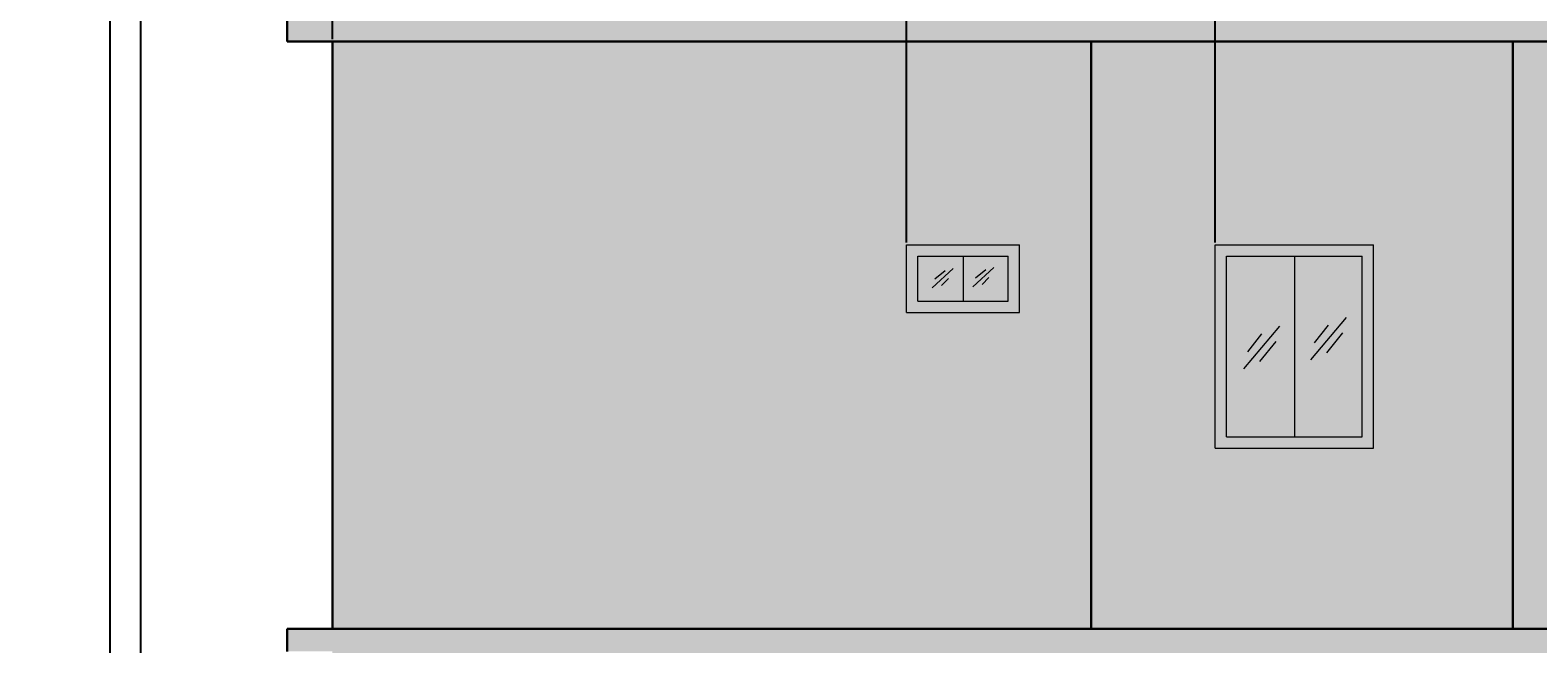
# Model space of a CAD drawing. Units: inches. Extents: x 2391 to 16591, y 7259 to 10239.
# Tile 14 of 27: x 3487 to 3888, y 8066 to 8229. Entities that reach past the tile are written whole.
import ezdxf

# ---------------------------------------------------------------- set-up
doc = ezdxf.new("R2010")
doc.units = ezdxf.units.IN
for name, color, linetype, lineweight in [('A-ANNO-DIMS', 4, 'Continuous', 18), ('A-ELEV', 7, 'Continuous', 30), ('A-ELEV-GLAZ', 4, 'Continuous', 18), ('A-ELEV-GLAZ-PATT', 141, 'Continuous', 13), ('A-ELEV-PATT', 8, 'Continuous', 13), ('A-ELEV-SURF-PATT', 253, 'Continuous', 13)]:
    doc.layers.add(name, color=color, linetype=linetype, lineweight=lineweight)
doc.styles.get("Standard").update_dxf_attribs({"font": 'arial.ttf'})
doc.dimstyles.new('ISO-25', dxfattribs={"dimtxt": 2.5, "dimasz": 2.5, "dimexe": 1.25, "dimexo": 0.625, "dimtad": 1, "dimdec": 0, "dimlunit": 3, "dimtxsty": 'Standard', "dimcen": 2.5, "dimadec": 0, "dimazin": 0, "dimtfac": 1, "dimtdec": 0, "dimtmove": 0, "dimatfit": 3, "dimfxl": 1, "dimarcsym": 0})

# ---------------------------------------------------------------- blocks, each defined once
blk = doc.blocks.new('GLASS-REFLECTION-VENT')
for p, q in [((0, 0), (5.55, 5.12)), ((0.7, 2.37), (3.45, 4.58)), ((2.48, 0.59), (4.26, 2.48))]:
    blk.add_line(p, q)
blk = doc.blocks.new('GLASS-REFLECTION-WINDOW')
for p, q in [((0, 0), (9.5, 11.3)), ((1, 4.52), (4.76, 9.26)), ((4.26, 1.91), (8.52, 7.21))]:
    blk.add_line(p, q)
blk = doc.blocks.new('*D84')
at = {"layer": 'A-ANNO-DIMS', "color": 0, "lineweight": -2, "transparency": 16777216}
for p, q in [((3437.4, 8339.52), (3518.08, 8339.52)), ((3516.83, 7579.02), (3516.83, 8337.02)), ((3464.4, 7576.52), (3518.08, 7576.52))]:
    blk.add_line(p, q, dxfattribs=at)
at = {"layer": 'A-ANNO-DIMS', "color": 0, "transparency": 16777216}
for points in [[(3516.41, 8337.02), (3517.24, 8337.02), (3516.83, 8339.52)], [(3516.41, 7579.02), (3517.24, 7579.02), (3516.83, 7576.52)]]:
    blk.add_solid(points, dxfattribs=at)
at = {"layer": 'Defpoints', "color": 0, "transparency": 16777216}
for p in [(3436.78, 8339.52), (3516.83, 8339.52), (3463.78, 7576.52)]:
    blk.add_point(p, dxfattribs=at)
at = {"layer": 'A-ANNO-DIMS', "color": 0, "transparency": 16777216, "insert": (3514.93, 7958.02), "char_height": 2.5, "attachment_point": 5, "rotation": 90}
blk.add_mtext('63\'-7"', dxfattribs=at)
blk = doc.blocks.new('*D92')
at = {"layer": 'A-ANNO-DIMS', "color": 0, "lineweight": -2, "transparency": 16777216}
for p, q in [((3777.58, 8333.18), (3507.41, 8333.18)), ((3508.66, 7572.68), (3508.66, 8330.68)), ((3561.08, 7570.18), (3507.41, 7570.18))]:
    blk.add_line(p, q, dxfattribs=at)
at = {"layer": 'A-ANNO-DIMS', "color": 0, "transparency": 16777216}
for points in [[(3508.24, 8330.68), (3509.08, 8330.68), (3508.66, 8333.18)], [(3508.24, 7572.68), (3509.08, 7572.68), (3508.66, 7570.18)]]:
    blk.add_solid(points, dxfattribs=at)
at = {"layer": 'Defpoints', "color": 0, "transparency": 16777216}
for p in [(3508.66, 8333.18), (3778.21, 8333.18), (3561.71, 7570.18)]:
    blk.add_point(p, dxfattribs=at)
at = {"layer": 'A-ANNO-DIMS', "color": 0, "transparency": 16777216, "insert": (3506.76, 7951.68), "char_height": 2.5, "attachment_point": 5, "rotation": 90}
blk.add_mtext('63\'-7"', dxfattribs=at)
blk = doc.blocks.new('*D93')
at = {"layer": 'A-ANNO-DIMS', "color": 0, "lineweight": -2, "transparency": 16777216}
for p, q in [((3567.71, 8226.81), (3567.71, 8381.48)), ((3570.21, 8380.23), (3717.71, 8380.23)), ((3720.21, 8172.81), (3720.21, 8381.48))]:
    blk.add_line(p, q, dxfattribs=at)
at = {"layer": 'A-ANNO-DIMS', "color": 0, "transparency": 16777216}
for points in [[(3570.21, 8380.65), (3570.21, 8379.81), (3567.71, 8380.23)], [(3717.71, 8380.65), (3717.71, 8379.81), (3720.21, 8380.23)]]:
    blk.add_solid(points, dxfattribs=at)
at = {"layer": 'Defpoints', "color": 0, "transparency": 16777216}
for p in [(3720.21, 8380.23), (3567.71, 8226.18), (3720.21, 8172.18)]:
    blk.add_point(p, dxfattribs=at)
at = {"layer": 'A-ANNO-DIMS', "color": 0, "transparency": 16777216, "insert": (3643.96, 8382.15), "char_height": 2.5, "attachment_point": 5}
blk.add_mtext('12\'-8 1/2"', dxfattribs=at)
blk = doc.blocks.new('*D94')
at = {"layer": 'A-ANNO-DIMS', "color": 0, "lineweight": -2, "transparency": 16777216}
for p, q in [((3720.21, 8172.81), (3720.21, 8381.48)), ((3722.71, 8380.23), (3799.71, 8380.23)), ((3802.21, 8172.81), (3802.21, 8381.48))]:
    blk.add_line(p, q, dxfattribs=at)
at = {"layer": 'A-ANNO-DIMS', "color": 0, "transparency": 16777216}
for points in [[(3722.71, 8380.65), (3722.71, 8379.81), (3720.21, 8380.23)], [(3799.71, 8380.65), (3799.71, 8379.81), (3802.21, 8380.23)]]:
    blk.add_solid(points, dxfattribs=at)
at = {"layer": 'Defpoints', "color": 0, "transparency": 16777216}
for p in [(3802.21, 8380.23), (3720.21, 8172.18), (3802.21, 8172.18)]:
    blk.add_point(p, dxfattribs=at)
at = {"layer": 'A-ANNO-DIMS', "color": 0, "transparency": 16777216, "insert": (3761.21, 8382.13), "char_height": 2.5, "attachment_point": 5}
blk.add_mtext('6\'-10"', dxfattribs=at)
blk = doc.blocks.new('*D95')
at = {"layer": 'A-ANNO-DIMS', "color": 0, "lineweight": -2, "transparency": 16777216}
for p, q in [((3802.21, 8172.81), (3802.21, 8381.48)), ((3804.71, 8380.23), (3912.46, 8380.23)), ((3914.96, 8172.81), (3914.96, 8381.48))]:
    blk.add_line(p, q, dxfattribs=at)
at = {"layer": 'A-ANNO-DIMS', "color": 0, "transparency": 16777216}
for points in [[(3804.71, 8380.65), (3804.71, 8379.81), (3802.21, 8380.23)], [(3912.46, 8380.65), (3912.46, 8379.81), (3914.96, 8380.23)]]:
    blk.add_solid(points, dxfattribs=at)
at = {"layer": 'Defpoints', "color": 0, "transparency": 16777216}
for p in [(3914.96, 8380.23), (3802.21, 8172.18), (3914.96, 8172.18)]:
    blk.add_point(p, dxfattribs=at)
at = {"layer": 'A-ANNO-DIMS', "color": 0, "transparency": 16777216, "insert": (3858.58, 8382.13), "char_height": 2.5, "attachment_point": 5}
blk.add_mtext('9\'-5"', dxfattribs=at)

msp = doc.modelspace()

# ---------------------------------------------------------------- hatches: boundary and pattern name
at = {"layer": 'A-ELEV-GLAZ-PATT'}
h = msp.add_hatch(color=256, dxfattribs=at)
h.dxf.hatch_style = 1
h.paths.add_polyline_path([(3750.21, 8172.18), (3720.21, 8172.18), (3720.21, 8154.18), (3750.21, 8154.18)])
h.paths.add_polyline_path([(3747.21, 8169.18), (3747.21, 8157.18), (3723.21, 8157.18), (3723.21, 8169.18)], flags=16)
h.paths.add_polyline_path([(3802.21, 8172.18), (3802.21, 8118.18), (3844.21, 8118.18), (3844.21, 8172.18)])
h.paths.add_polyline_path([(3841.21, 8169.18), (3841.21, 8121.18), (3805.21, 8121.18), (3805.21, 8169.18)], flags=16)
h.paths.add_polyline_path([(3956.96, 8172.18), (3914.96, 8172.18), (3914.96, 8118.18), (3956.96, 8118.18)])
h.paths.add_polyline_path([(3953.96, 8169.18), (3953.96, 8121.18), (3917.96, 8121.18), (3917.96, 8169.18)], flags=16)
h.paths.add_polyline_path([(3720.21, 8010.18), (3720.21, 7992.18), (3750.21, 7992.18), (3750.21, 8010.18)])
h.paths.add_polyline_path([(3747.21, 8007.18), (3747.21, 7995.18), (3723.21, 7995.18), (3723.21, 8007.18)], flags=16)
h.paths.add_polyline_path([(3802.21, 8010.18), (3802.21, 7956.18), (3844.21, 7956.18), (3844.21, 8010.18)])
h.paths.add_polyline_path([(3841.21, 8007.18), (3841.21, 7959.18), (3805.21, 7959.18), (3805.21, 8007.18)], flags=16)
h.paths.add_polyline_path([(3914.96, 8010.18), (3914.96, 7956.18), (3956.96, 7956.18), (3956.96, 8010.18)])
h.paths.add_polyline_path([(3917.96, 8007.18), (3953.96, 8007.18), (3953.96, 7959.18), (3917.96, 7959.18)], flags=16)
h.paths.add_polyline_path([(3750.21, 7848.18), (3720.21, 7848.18), (3720.21, 7830.18), (3750.21, 7830.18)])
h.paths.add_polyline_path([(3747.21, 7845.18), (3747.21, 7833.18), (3723.21, 7833.18), (3723.21, 7845.18)], flags=16)
h.paths.add_polyline_path([(3844.21, 7848.18), (3802.21, 7848.18), (3802.21, 7794.18), (3844.21, 7794.18)])
h.paths.add_polyline_path([(3805.21, 7845.18), (3841.21, 7845.18), (3841.21, 7797.18), (3805.21, 7797.18)], flags=16)
h.paths.add_polyline_path([(3914.96, 7848.18), (3914.96, 7794.18), (3956.96, 7794.18), (3956.96, 7848.18)])
h.paths.add_polyline_path([(3917.96, 7845.18), (3953.96, 7845.18), (3953.96, 7797.18), (3917.96, 7797.18)], flags=16)
h = msp.add_hatch(color=256, dxfattribs=at)
h.dxf.hatch_style = 1
h.paths.add_polyline_path([(3735.21, 8169.18), (3723.21, 8169.18), (3723.21, 8157.18), (3735.21, 8157.18)])
h.paths.add_polyline_path([(3747.21, 8169.18), (3735.21, 8169.18), (3735.21, 8157.18), (3747.21, 8157.18)])
h.paths.add_polyline_path([(3823.21, 8169.18), (3805.21, 8169.18), (3805.21, 8121.18), (3823.21, 8121.18)])
h.paths.add_polyline_path([(3841.21, 8169.18), (3823.21, 8169.18), (3823.21, 8121.18), (3841.21, 8121.18)])
h.paths.add_polyline_path([(3935.96, 8169.18), (3917.96, 8169.18), (3917.96, 8121.18), (3935.96, 8121.18)])
h.paths.add_polyline_path([(3953.96, 8169.18), (3935.96, 8169.18), (3935.96, 8121.18), (3953.96, 8121.18)])
h.paths.add_polyline_path([(3735.21, 8007.18), (3723.21, 8007.18), (3723.21, 7995.18), (3735.21, 7995.18)])
h.paths.add_polyline_path([(3747.21, 8007.18), (3735.21, 8007.18), (3735.21, 7995.18), (3747.21, 7995.18)])
h.paths.add_polyline_path([(3823.21, 8007.18), (3805.21, 8007.18), (3805.21, 7959.18), (3823.21, 7959.18)])
h.paths.add_polyline_path([(3841.21, 8007.18), (3823.21, 8007.18), (3823.21, 7959.18), (3841.21, 7959.18)])
h.paths.add_polyline_path([(3935.96, 8007.18), (3917.96, 8007.18), (3917.96, 7959.18), (3935.96, 7959.18)])
h.paths.add_polyline_path([(3953.96, 8007.18), (3935.96, 8007.18), (3935.96, 7959.18), (3953.96, 7959.18)])
h.paths.add_polyline_path([(3735.21, 7845.18), (3723.21, 7845.18), (3723.21, 7833.18), (3735.21, 7833.18)])
h.paths.add_polyline_path([(3747.21, 7845.18), (3735.21, 7845.18), (3735.21, 7833.18), (3747.21, 7833.18)])
h.paths.add_polyline_path([(3823.21, 7845.18), (3805.21, 7845.18), (3805.21, 7797.18), (3823.21, 7797.18)])
h.paths.add_polyline_path([(3841.21, 7845.18), (3823.21, 7845.18), (3823.21, 7797.18), (3841.21, 7797.18)])
h.paths.add_polyline_path([(3935.96, 7845.18), (3917.96, 7845.18), (3917.96, 7797.18), (3935.96, 7797.18)])
h.paths.add_polyline_path([(3953.96, 7845.18), (3935.96, 7845.18), (3935.96, 7797.18), (3953.96, 7797.18)])
at = {"layer": 'A-ELEV-PATT'}
h = msp.add_hatch(dxfattribs=at)
h.set_pattern_fill('BRSTONE', color=256)
h.paths.add_polyline_path([(3999.71, 8226.18), (3881.21, 8226.18), (3881.21, 8070.18), (3999.71, 8070.18)])
h.paths.add_polyline_path([(3956.96, 8118.18), (3914.96, 8118.18), (3914.96, 8172.18), (3956.96, 8172.18)], flags=16)
h.paths.add_polyline_path([(3953.96, 8121.18), (3917.96, 8121.18), (3917.96, 8169.18), (3953.96, 8169.18)], flags=0)
h.paths.add_polyline_path([(3999.71, 8064.18), (3881.21, 8064.18), (3881.21, 7908.18), (3999.71, 7908.18)])
h.paths.add_polyline_path([(3956.96, 7956.18), (3914.96, 7956.18), (3914.96, 8010.18), (3956.96, 8010.18)], flags=16)
h.paths.add_polyline_path([(3953.96, 7959.18), (3917.96, 7959.18), (3917.96, 8007.18), (3953.96, 8007.18)], flags=0)
h.paths.add_polyline_path([(3999.71, 7902.18), (3881.21, 7902.18), (3881.21, 7746.18), (3999.71, 7746.18)])
h.paths.add_polyline_path([(3956.96, 7794.18), (3914.96, 7794.18), (3914.96, 7848.18), (3956.96, 7848.18)], flags=16)
h.paths.add_polyline_path([(3953.96, 7797.18), (3917.96, 7797.18), (3917.96, 7845.18), (3953.96, 7845.18)], flags=0)
h.paths.add_polyline_path([(3999.71, 7740.18), (3567.71, 7740.18), (3567.71, 7697.18), (3760.71, 7697.18), (3760.71, 7706.18), (3755.71, 7706.18), (3755.71, 7711.18), (3774.71, 7711.18), (3774.71, 7706.18), (3769.71, 7706.18), (3769.71, 7677.02), (3772.21, 7677.02), (3772.21, 7679.02), (3774.71, 7679.02), (3774.71, 7704.18), (3843.71, 7704.18), (3843.71, 7589.18), (3774.71, 7589.18), (3774.71, 7584.18), (3913.71, 7584.18), (3913.71, 7589.18), (3844.71, 7589.18), (3844.71, 7704.18), (3913.71, 7704.18), (3913.71, 7679.02), (3916.21, 7679.02), (3916.21, 7677.02), (3918.71, 7677.02), (3918.71, 7706.18), (3913.71, 7706.18), (3913.71, 7711.18), (3932.71, 7711.18), (3932.71, 7706.18), (3927.71, 7706.18), (3927.71, 7697.18), (3999.71, 7697.18)])
h.paths.add_polyline_path([(3918.71, 7675.02), (3916.21, 7675.02), (3916.21, 7673.02), (3913.71, 7673.02), (3913.71, 7618.89), (3916.21, 7618.89), (3916.21, 7616.89), (3918.71, 7616.89)], flags=17)
h.paths.add_polyline_path([(3918.71, 7614.89), (3916.21, 7614.89), (3916.21, 7612.89), (3913.71, 7612.89), (3913.71, 7584.18), (3918.71, 7584.18)], flags=17)
h.paths.add_polyline_path([(3774.71, 7673.02), (3772.21, 7673.02), (3772.21, 7675.02), (3769.71, 7675.02), (3769.71, 7616.89), (3772.21, 7616.89), (3772.21, 7618.89), (3774.71, 7618.89)], flags=17)
h.paths.add_polyline_path([(3774.71, 7612.89), (3772.21, 7612.89), (3772.21, 7614.89), (3769.71, 7614.89), (3769.71, 7584.18), (3774.71, 7584.18), (3774.71, 7589.18)], flags=17)
h = msp.add_hatch(dxfattribs=at)
h.set_pattern_fill('GRAVEL', color=256)
h.paths.add_polyline_path([(3769.21, 8226.18), (3567.71, 8226.18), (3567.71, 8070.18), (3769.21, 8070.18)])
h.paths.add_polyline_path([(3720.21, 8154.18), (3720.21, 8172.18), (3750.21, 8172.18), (3750.21, 8154.18)], flags=16)
h.paths.add_polyline_path([(3723.21, 8157.18), (3723.21, 8169.18), (3747.21, 8169.18), (3747.21, 8157.18)], flags=0)
h.paths.add_polyline_path([(3769.21, 8064.18), (3567.71, 8064.18), (3567.71, 7908.18), (3769.21, 7908.18)])
h.paths.add_polyline_path([(3720.21, 7992.18), (3720.21, 8010.18), (3750.21, 8010.18), (3750.21, 7992.18)], flags=16)
h.paths.add_polyline_path([(3723.21, 7995.18), (3723.21, 8007.18), (3747.21, 8007.18), (3747.21, 7995.18)], flags=0)
h.paths.add_polyline_path([(3769.21, 7902.18), (3567.71, 7902.18), (3567.71, 7746.18), (3769.21, 7746.18)])
h.paths.add_polyline_path([(3720.21, 7848.18), (3750.21, 7848.18), (3750.21, 7830.18), (3720.21, 7830.18)], flags=16)
h.paths.add_polyline_path([(3723.21, 7845.18), (3747.21, 7845.18), (3747.21, 7833.18), (3723.21, 7833.18)], flags=0)
h = msp.add_hatch(dxfattribs=at)
h.set_pattern_fill('HONEY', color=256)
h.paths.add_polyline_path([(3881.21, 8226.18), (3769.21, 8226.18), (3769.21, 8070.18), (3881.21, 8070.18)])
h.paths.add_polyline_path([(3844.21, 8118.18), (3802.21, 8118.18), (3802.21, 8172.18), (3844.21, 8172.18)], flags=16)
h.paths.add_polyline_path([(3841.21, 8121.18), (3805.21, 8121.18), (3805.21, 8169.18), (3841.21, 8169.18)], flags=0)
h.paths.add_polyline_path([(3881.21, 8064.18), (3769.21, 8064.18), (3769.21, 7908.18), (3881.21, 7908.18)])
h.paths.add_polyline_path([(3844.21, 7956.18), (3802.21, 7956.18), (3802.21, 8010.18), (3844.21, 8010.18)], flags=16)
h.paths.add_polyline_path([(3841.21, 7959.18), (3805.21, 7959.18), (3805.21, 8007.18), (3841.21, 8007.18)], flags=0)
h.paths.add_polyline_path([(3881.21, 7902.18), (3769.21, 7902.18), (3769.21, 7746.18), (3881.21, 7746.18)])
h.paths.add_polyline_path([(3844.21, 7794.18), (3802.21, 7794.18), (3802.21, 7848.18), (3844.21, 7848.18)], flags=16)
h.paths.add_polyline_path([(3841.21, 7797.18), (3805.21, 7797.18), (3805.21, 7845.18), (3841.21, 7845.18)], flags=0)
at = {"layer": 'A-ELEV-SURF-PATT'}
h = msp.add_hatch(color=256, dxfattribs=at)
h.dxf.hatch_style = 1
h.paths.add_polyline_path([(4011.71, 7740.18), (4011.71, 7746.18), (3555.71, 7746.18), (3555.71, 7740.18)])
h.paths.add_polyline_path([(4011.71, 7902.18), (4011.71, 7908.18), (3555.71, 7908.18), (3555.71, 7902.18)])
h.paths.add_polyline_path([(4011.71, 8064.18), (4011.71, 8070.18), (3555.71, 8070.18), (3555.71, 8064.18)])
h.paths.add_polyline_path([(3555.71, 8232.18), (3555.71, 8226.18), (4011.71, 8226.18), (4011.71, 8232.18)])
h.paths.add_polyline_path([(3778.21, 8333.18), (3778.21, 8328.18), (3978.71, 8328.18), (3978.71, 8333.18)])

# ---------------------------------------------------------------- linework, layer by layer
at = {"layer": 'A-ELEV'}
for p, q in [((3555.71, 8226.18), (3555.71, 8232.18)), ((3555.71, 8226.18), (4011.71, 8226.18)), ((3567.71, 8070.18), (3567.71, 8226.18)), ((3769.21, 8226.18), (3769.21, 8070.18)), ((3881.21, 8226.18), (3881.21, 8070.18)), ((3555.71, 8064.18), (3555.71, 8070.18)), ((3555.71, 8070.18), (4011.71, 8070.18))]:
    msp.add_line(p, q, dxfattribs=at)
at = {"layer": 'A-ELEV-GLAZ'}
for p, q in [((3720.21, 8172.18), (3750.21, 8172.18)), ((3720.21, 8154.18), (3720.21, 8172.18)), ((3750.21, 8154.18), (3750.21, 8172.18)), ((3802.21, 8172.18), (3844.21, 8172.18)), ((3802.21, 8118.18), (3802.21, 8172.18)), ((3844.21, 8118.18), (3844.21, 8172.18)), ((3723.21, 8169.18), (3747.21, 8169.18)), ((3723.21, 8157.18), (3723.21, 8169.18)), ((3735.21, 8169.18), (3735.21, 8157.18)), ((3747.21, 8157.18), (3747.21, 8169.18)), ((3805.21, 8169.18), (3841.21, 8169.18)), ((3805.21, 8121.18), (3805.21, 8169.18)), ((3823.21, 8169.18), (3823.21, 8121.18)), ((3841.21, 8121.18), (3841.21, 8169.18)), ((3720.21, 8154.18), (3750.21, 8154.18)), ((3723.21, 8157.18), (3747.21, 8157.18)), ((3802.21, 8118.18), (3844.21, 8118.18)), ((3805.21, 8121.18), (3841.21, 8121.18))]:
    msp.add_line(p, q, dxfattribs=at)

# ---------------------------------------------------------------- block references
for name, p in [('GLASS-REFLECTION-VENT', (3727.04, 8160.76)), ('GLASS-REFLECTION-VENT', (3737.79, 8161.04)), ('GLASS-REFLECTION-WINDOW', (3809.81, 8139.25)), ('GLASS-REFLECTION-WINDOW', (3827.54, 8141.6))]:
    msp.add_blockref(name, p, dxfattribs=at)

# ---------------------------------------------------------------- dimensions: what is measured, and where the dimension line sits
at = {"layer": 'A-ANNO-DIMS'}
for base, p1, p2, picture, middle in [((3720.21, 8380.23), (3567.71, 8226.18), (3720.21, 8172.18), '*D93', (3643.96, 8382.15)), ((3802.21, 8380.23), (3720.21, 8172.18), (3802.21, 8172.18), '*D94', (3761.21, 8382.13)), ((3914.959246, 8380.230453), (3802.209246, 8172.180453), (3914.959246, 8172.180453), '*D95', (3858.584246, 8382.13188547))]:
    dim = msp.add_linear_dim(base=base, p1=p1, p2=p2, dimstyle='ISO-25', override={"dimdec": 1, "dimlfac": 1, "dimrnd": 0, "dimzin": 1, "dimdsep": 46, "dimlunit": 4, "dimfrac": 2}, dxfattribs=at)
    dim.commit()
    dim.dimension.update_dxf_attribs({"geometry": picture, "text_midpoint": middle})
for base, p1, p2, picture, middle in [((3516.83, 8339.52), (3463.78, 7576.52), (3436.78, 8339.52), '*D84', (3514.93, 7958.02)), ((3508.66, 8333.18), (3561.71, 7570.18), (3778.21, 8333.18), '*D92', (3506.76, 7951.68))]:
    dim = msp.add_linear_dim(base=base, p1=p1, p2=p2, angle=90, dimstyle='ISO-25', override={"dimdec": 1, "dimlfac": 1, "dimrnd": 0, "dimzin": 1, "dimdsep": 46, "dimlunit": 4, "dimfrac": 2}, dxfattribs=at)
    dim.commit()
    dim.dimension.update_dxf_attribs({"geometry": picture, "text_midpoint": middle})

doc.saveas('drawing.dxf')
